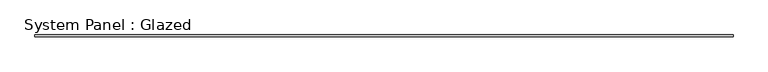
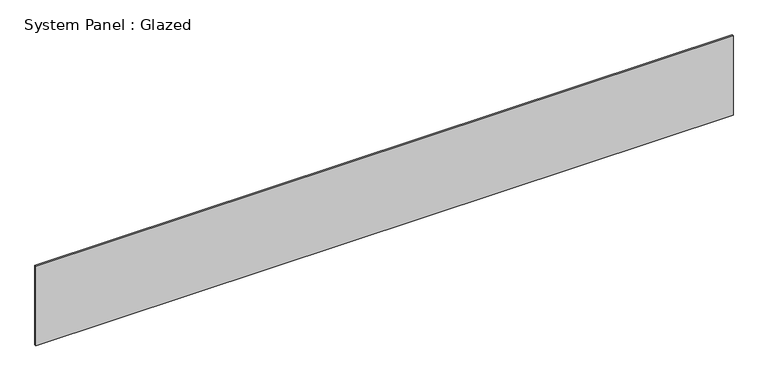
"""IFC4 building model written with IfcOpenShell, lengths in millimetres: plate geometry, System Panel : Glazed."""

from ifc_helpers import new_model, si_unit, origin, origin_with_axes, place, context, project, spatial, polyline, outline, extrude, source, transform, mapped, element, save


def system_panel_glazed_f39c722f(model_context):
    return source(origin(), model_context, "Body", "SweptSolid", [
        extrude(outline(polyline([(5067.3, 19.05), (-5067.3, 19.05), (-5067.3, 44.45), (5067.3, 44.45), (5067.3, 19.05)])), origin_with_axes(), (0.0, 0.0, 1.0), 1219.2),
    ])


if __name__ == "__main__":
    model = new_model("IFC4")
    model_context = context("Model", 3, world=origin())
    ifc_project = project(units=[si_unit("LENGTHUNIT", "METRE", prefix="MILLI")], contexts=[model_context])
    site = spatial("IfcSite", under=ifc_project)
    building = spatial("IfcBuilding", under=site)
    placement = place(None, origin())
    system_panel_glazed_shape = system_panel_glazed_f39c722f(model_context)
    element("IfcPlate", 1, ObjectType="System Panel : Glazed", at=placement, inside=building, context=model_context, shape_type="MappedRepresentation", body=[
        mapped(system_panel_glazed_shape, transform((0.0, 0.0, 0.0), x_axis=(1.0, 0.0, 0.0), y_axis=(0.0, 1.0, 0.0), z_axis=(0.0, 0.0, 1.0))),
    ])
    save(model, "model.ifc")

# Revit data of these elements
# Type "System Panel : Glazed"
#   Construction Type Id = "GSP4R"
#   Analytic Construction = "1/8 in Pilkington single glazing"
#   Visual Light Transmittance = 0.9
#   Solar Heat Gain Coefficient = 0.86
#   Heat Transfer Coefficient (U) = 1.18115 BTU/(h·ft²·°F)
# Element 1 (IfcPlate, "System Panel : Glazed")
#   Materials on its faces: "Glass"
# Materials
#   "Glass": class "Glass", colour RGB 0 128 192, transparency 0.75, Description = "Soda Lime Glass", Cost = 0
